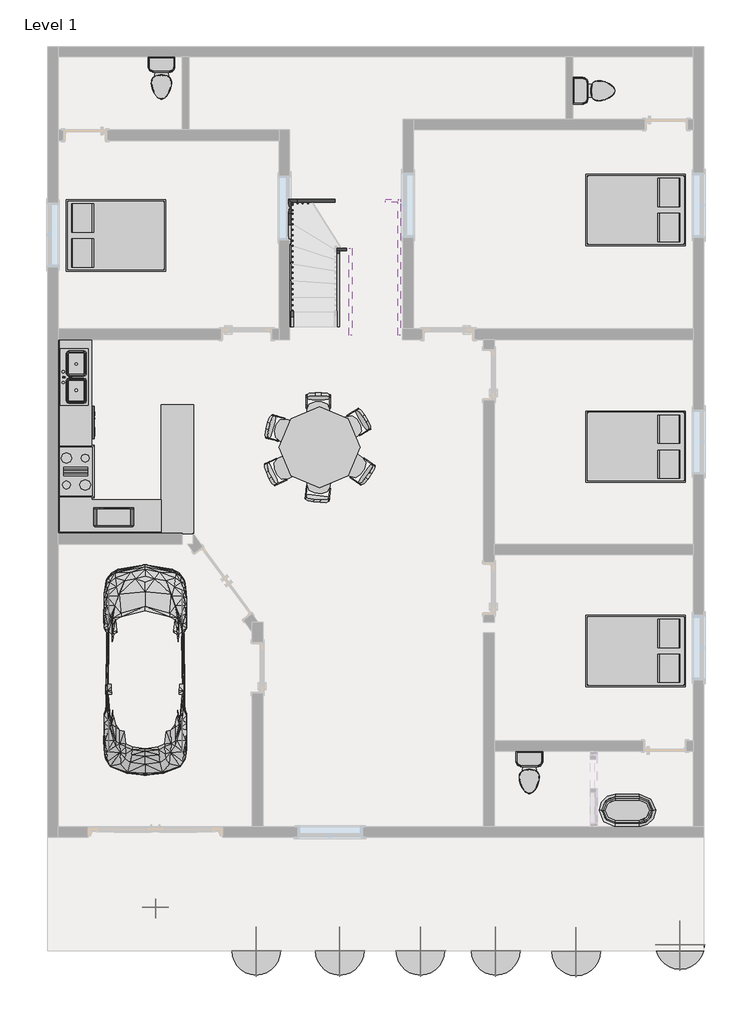
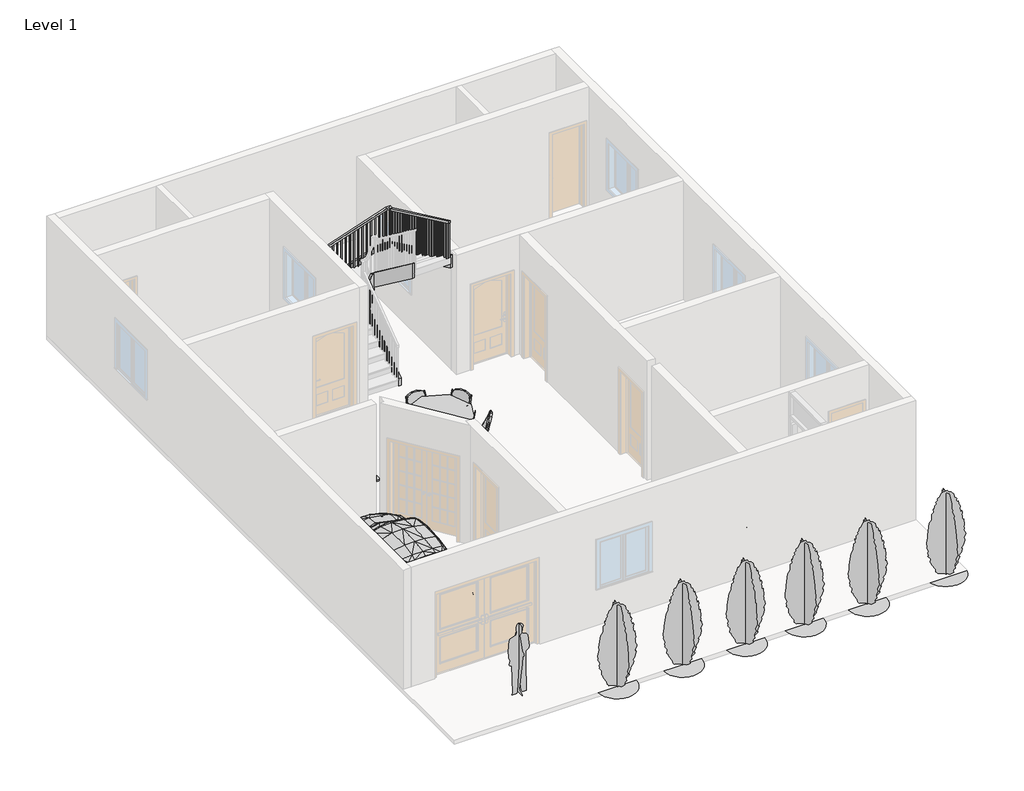
# One storey, part 3 of 3: 13 furniture elements, 9 members, 6 geographic elements, 5 flow terminals, 5 proxies, 1 railing.
"""IFC4 building model written with IfcOpenShell, lengths in millimetres."""

from ifc_helpers import new_model, si_unit, frame, origin, place, context, project, spatial, polyline, outline, extrude, faceted_brep, transform, mapped, element, save
from components import proxy_bb1e6e30, proxy_45b28599, proxy_487063f8, rpc_beetle_rpc_beetle_3ce7ba48, rpc_male_28878092, flow_terminal_a53be723, toilet_domestic_3d_toilet_domestic_3d_f7549cf7, toilet_domestic_3d_toilet_domestic_3d_183bbd19, flow_terminal_f143e1fa, furniture_c8abb964, furniture_15b2fe13, furniture_067af109, furniture_3d1d9cbc, furniture_720490b2, rpc_tree_conifer_chinese_juniper_7_1b9786cd

model = new_model("IFC4")

# Units and contexts
model_context = context("Model", 3, world=origin())
ifc_project = project(units=[si_unit("LENGTHUNIT", "METRE", prefix="MILLI")], contexts=[model_context])

# Site, building, storey
site = spatial("IfcSite", under=ifc_project)
building = spatial("IfcBuilding", under=site)
storey = spatial("IfcBuildingStorey", under=building, Name="Level 1", Elevation=0.0)

# Proxies
placement = place(None, origin())
proxy_shape = proxy_bb1e6e30(model_context)
element("IfcBuildingElementProxy", 1, Name="Cook Top-4 Unit.0001 : 36\" x 20\"", ObjectType="Cook Top-4 Unit.0001 : 36\" x 20\"", at=placement, inside=storey, context=model_context, shape_type="MappedRepresentation", body=[
    mapped(proxy_shape, transform((-2044.8374747, 336.6527309, 152.4), x_axis=(0.0, 1.0, 0.0), y_axis=(-1.0, 0.0, 0.0), z_axis=(0.0, 0.0, 1.0))),
])
proxy_2_shape = proxy_45b28599(model_context)
element("IfcBuildingElementProxy", 2, Name="Dishwasher : 24\" x 24\" x 34\"", ObjectType="Dishwasher : 24\" x 24\" x 34\"", at=placement, inside=storey, context=model_context, shape_type="MappedRepresentation", body=[
    mapped(proxy_2_shape, transform((-1744.7999747, 882.7527309, 0.0), x_axis=(0.0, 1.000000000000002, 0.0), y_axis=(-1.000000000000002, 0.0, 0.0), z_axis=(0.0, 0.0, 1.0))),
])
proxy_3_shape = proxy_487063f8(model_context)
element("IfcBuildingElementProxy", 3, Name="Microwave : 30\" x 16\" x 18\"", ObjectType="Microwave : 30\" x 16\" x 18\"", at=placement, inside=storey, context=model_context, shape_type="MappedRepresentation", body=[
    mapped(proxy_3_shape, transform((-828.5820974, -880.0277749, 0.0), x_axis=(-1.0000000000000004, 0.0, 0.0), y_axis=(0.0, -1.0000000000000004, 0.0), z_axis=(0.0, 0.0, 1.0))),
])
rpc_beetle_rpc_beetle_shape = rpc_beetle_rpc_beetle_3ce7ba48(model_context)
element("IfcBuildingElementProxy", 4, Name="RPC Beetle : RPC Beetle", ObjectType="RPC Beetle : RPC Beetle", at=placement, inside=storey, context=model_context, shape_type="MappedRepresentation", body=[
    mapped(rpc_beetle_rpc_beetle_shape, transform((-731.9749747, -4641.7472691, 0.0), x_axis=(1.0, 0.0, 0.0), y_axis=(0.0, 1.0, 0.0), z_axis=(0.0, 0.0, 1.0))),
])
rpc_male_shape = rpc_male_28878092(model_context)
element("IfcBuildingElementProxy", 5, Name="RPC Male", ObjectType="RPC Male", at=placement, inside=storey, context=model_context, shape_type="MappedRepresentation", body=[
    mapped(rpc_male_shape, transform((-545.8247746, -7892.9472691, 0.0), x_axis=(1.0, 0.0, 0.0), y_axis=(0.0, 1.0, 0.0), z_axis=(0.0, 0.0, 1.0))),
])

# Flow terminals
flow_terminal_shape = flow_terminal_a53be723(model_context)
element("IfcFlowTerminal", 6, ObjectType="Sink Kitchen-Double : 42\" x 21\"", at=placement, inside=storey, context=model_context, shape_type="MappedRepresentation", body=[
    mapped(flow_terminal_shape, transform((-2072.3615606, 2103.7489712, 30.4601563), x_axis=(0.0, 1.0000000000000002, 0.0), y_axis=(-1.0000000000000002, 0.0, 0.0), z_axis=(0.0, 0.0, 1.0))),
])
toilet_domestic_3d_toilet_domestic_3d_shape = toilet_domestic_3d_toilet_domestic_3d_f7549cf7(model_context)
toilet_domestic_3d_toilet_domestic_3d_2_shape = toilet_domestic_3d_toilet_domestic_3d_183bbd19(model_context)
element("IfcFlowTerminal", 7, ObjectType="Toilet-Domestic-3D : Toilet-Domestic-3D", at=placement, inside=storey, context=model_context, shape_type="MappedRepresentation", body=[
    mapped(toilet_domestic_3d_toilet_domestic_3d_shape, transform((-427.1749747, 7674.6817036, 0.0), x_axis=(1.0, 0.0, 0.0), y_axis=(0.0, 1.0, 0.0), z_axis=(0.0, 0.0, 1.0))),
    mapped(toilet_domestic_3d_toilet_domestic_3d_2_shape, transform((-427.1749747, 7674.6817036, 0.0), x_axis=(1.0, 0.0, 0.0), y_axis=(0.0, 1.0, 0.0), z_axis=(0.0, 0.0, 1.0))),
])
element("IfcFlowTerminal", 8, ObjectType="Toilet-Domestic-3D : Toilet-Domestic-3D", at=placement, inside=storey, context=model_context, shape_type="MappedRepresentation", body=[
    mapped(toilet_domestic_3d_toilet_domestic_3d_shape, transform((7839.9210527, 7527.3770127, 0.0), x_axis=(0.0, 1.0000000000000002, 0.0), y_axis=(-1.0000000000000002, 0.0, 0.0), z_axis=(0.0, 0.0, 1.0))),
    mapped(toilet_domestic_3d_toilet_domestic_3d_2_shape, transform((7839.9210527, 7527.3770127, 0.0), x_axis=(0.0, 1.0000000000000002, 0.0), y_axis=(-1.0000000000000002, 0.0, 0.0), z_axis=(0.0, 0.0, 1.0))),
])
element("IfcFlowTerminal", 9, ObjectType="Toilet-Domestic-3D : Toilet-Domestic-3D", at=placement, inside=storey, context=model_context, shape_type="MappedRepresentation", body=[
    mapped(toilet_domestic_3d_toilet_domestic_3d_shape, transform((6524.4875253, -5441.2432964, 0.0), x_axis=(1.0000000000000007, 0.0, 0.0), y_axis=(0.0, 1.0000000000000007, 0.0), z_axis=(0.0, 0.0, 1.0))),
    mapped(toilet_domestic_3d_toilet_domestic_3d_2_shape, transform((6524.4875253, -5441.2432964, 0.0), x_axis=(1.0000000000000007, 0.0, 0.0), y_axis=(0.0, 1.0000000000000007, 0.0), z_axis=(0.0, 0.0, 1.0))),
])
flow_terminal_2_shape = flow_terminal_f143e1fa(model_context)
element("IfcFlowTerminal", 10, ObjectType="Tub-Free Standing-3D : 30\" x 60\"", at=placement, inside=storey, context=model_context, shape_type="MappedRepresentation", body=[
    mapped(flow_terminal_2_shape, transform((8378.6875253, -6064.1472691, 0.0), x_axis=(0.0, 1.0000000000000002, 0.0), y_axis=(-1.0000000000000002, 0.0, 0.0), z_axis=(0.0, 0.0, 1.0))),
])

# Furniture
furniture_shape = furniture_c8abb964(model_context)
element("IfcFurniture", 11, ObjectType="Bed-Box : Double 53\" x 74\"", at=placement, inside=storey, context=model_context, shape_type="MappedRepresentation", body=[
    mapped(furniture_shape, transform((-1522.0294829, 4455.2002719, 0.0), x_axis=(0.0, 1.0, 0.0), y_axis=(-1.0, 0.0, 0.0), z_axis=(0.0, 0.0, 1.0))),
])
element("IfcFurniture", 12, ObjectType="Bed-Box : Double 53\" x 74\"", at=placement, inside=storey, context=model_context, shape_type="MappedRepresentation", body=[
    mapped(furniture_shape, transform((8770.2795335, 5616.10519, 0.0), x_axis=(0.0, -1.0000000000000004, 0.0), y_axis=(1.0000000000000004, 0.0, 0.0), z_axis=(0.0, 0.0, 1.0))),
])
element("IfcFurniture", 13, ObjectType="Bed-Box : Double 53\" x 74\"", at=placement, inside=storey, context=model_context, shape_type="MappedRepresentation", body=[
    mapped(furniture_shape, transform((8770.2795335, 1145.70519, 0.0), x_axis=(0.0, -1.0, 0.0), y_axis=(1.0, 0.0, 0.0), z_axis=(0.0, 0.0, 1.0))),
])
element("IfcFurniture", 14, ObjectType="Bed-Box : Double 53\" x 74\"", at=placement, inside=storey, context=model_context, shape_type="MappedRepresentation", body=[
    mapped(furniture_shape, transform((8770.2795335, -2711.3472691, 0.0), x_axis=(0.0, -1.0, 0.0), y_axis=(1.0, 0.0, 0.0), z_axis=(0.0, 0.0, 1.0))),
])
furniture_2_shape = furniture_15b2fe13(model_context)
element("IfcFurniture", 15, ObjectType="Counter Top-Island.0001 : 48\" Depth", at=placement, inside=storey, context=model_context, shape_type="MappedRepresentation", body=[
    mapped(furniture_2_shape, transform((-406.5374747, 364.407303, 30.4601563), x_axis=(0.0, 1.0000000000000002, 0.0), y_axis=(-1.0000000000000002, 0.0, 0.0), z_axis=(0.0, 0.0, 1.0))),
])
furniture_3_shape = furniture_067af109(model_context)
element("IfcFurniture", 16, ObjectType="Counter Top-L Shaped w Sink : 24\" Depth", at=placement, inside=storey, context=model_context, shape_type="MappedRepresentation", body=[
    mapped(furniture_3_shape, transform((-2379.7999747, 368.715026, 30.4601563), x_axis=(0.0, 1.0000000000000002, 0.0), y_axis=(-1.0000000000000002, 0.0, 0.0), z_axis=(0.0, 0.0, 1.0))),
])
furniture_4_shape = furniture_3d1d9cbc(model_context)
element("IfcFurniture", 17, ObjectType="Seating-Auditorium : 18\" x 24\" x 30\"", at=placement, inside=storey, context=model_context, shape_type="MappedRepresentation", body=[
    mapped(furniture_4_shape, transform((2361.6566068, -123.8075195, 0.0), x_axis=(0.9945218953682721, -0.10452846326766581, 0.0), y_axis=(0.1045284632676658, 0.994521895368272, 0.0), z_axis=(0.0, 0.0, 0.9999999999999999))),
])
element("IfcFurniture", 18, ObjectType="Seating-Auditorium : 18\" x 24\" x 30\"", at=placement, inside=storey, context=model_context, shape_type="MappedRepresentation", body=[
    mapped(furniture_4_shape, transform((3333.5819168, 167.1076408, 0.0), x_axis=(0.5790443741496127, 0.8152960276891364, 0.0), y_axis=(-0.8152960276891364, 0.5790443741496127, 0.0), z_axis=(0.0, 0.0, 1.0))),
])
element("IfcFurniture", 19, ObjectType="Seating-Auditorium : 18\" x 24\" x 30\"", at=placement, inside=storey, context=model_context, shape_type="MappedRepresentation", body=[
    mapped(furniture_4_shape, transform((1606.8827994, 449.404179, 0.0), x_axis=(0.42261826174068884, -0.9063077870366555, 0.0), y_axis=(0.9063077870366555, 0.42261826174068884, 0.0), z_axis=(0.0, 0.0, 1.0))),
])
element("IfcFurniture", 20, ObjectType="Seating-Auditorium : 18\" x 24\" x 30\"", at=placement, inside=storey, context=model_context, shape_type="MappedRepresentation", body=[
    mapped(furniture_4_shape, transform((1704.5988843, 1330.5740196, 0.0), x_axis=(-0.2588190451025253, -0.9659258262890678, 0.0), y_axis=(0.9659258262890678, -0.2588190451025253, 0.0), z_axis=(0.0, 0.0, 1.0))),
])
element("IfcFurniture", 21, ObjectType="Seating-Auditorium : 18\" x 24\" x 30\"", at=placement, inside=storey, context=model_context, shape_type="MappedRepresentation", body=[
    mapped(furniture_4_shape, transform((2697.4913996, 1720.3281408, 0.0), x_axis=(-1.0000000000000004, 0.0, 0.0), y_axis=(0.0, -1.0000000000000004, 0.0), z_axis=(0.0, 0.0, 1.0))),
])
element("IfcFurniture", 22, ObjectType="Seating-Auditorium : 18\" x 24\" x 30\"", at=placement, inside=storey, context=model_context, shape_type="MappedRepresentation", body=[
    mapped(furniture_4_shape, transform((3441.5258387, 1164.5071923, 0.0), x_axis=(-0.515038074910047, 0.8571673007021169, 0.0), y_axis=(-0.8571673007021169, -0.515038074910047, 0.0), z_axis=(0.0, 0.0, 1.0))),
])
furniture_5_shape = furniture_720490b2(model_context)
element("IfcFurniture", 23, ObjectType="Table-Dining Round : 36\" Diameter", at=placement, inside=storey, context=model_context, shape_type="MappedRepresentation", body=[
    mapped(furniture_5_shape, transform((2458.4815635, 978.7314195, 0.0), x_axis=(1.0, 0.0, 0.0), y_axis=(0.0, 1.0, 0.0), z_axis=(0.0, 0.0, 1.0))),
])

# Geographic elements
rpc_tree_conifer_chinese_juniper_7_shape = rpc_tree_conifer_chinese_juniper_7_1b9786cd(model_context)
element("IfcGeographicElement", 24, ObjectType="RPC Tree - Conifer : Chinese Juniper - 7'", at=placement, inside=storey, context=model_context, shape_type="MappedRepresentation", body=[
    mapped(rpc_tree_conifer_chinese_juniper_7_shape, transform((1362.8984947, -8713.8662612, 0.0), x_axis=(1.0, 0.0, 0.0), y_axis=(0.0, 1.0, 0.0), z_axis=(0.0, 0.0, 1.0))),
])
element("IfcGeographicElement", 25, ObjectType="RPC Tree - Conifer : Chinese Juniper - 7'", at=placement, inside=storey, context=model_context, shape_type="MappedRepresentation", body=[
    mapped(rpc_tree_conifer_chinese_juniper_7_shape, transform((2942.5370001, -8713.8662612, 0.0), x_axis=(1.0, 0.0, 0.0), y_axis=(0.0, 1.0, 0.0), z_axis=(0.0, 0.0, 1.0))),
])
element("IfcGeographicElement", 26, ObjectType="RPC Tree - Conifer : Chinese Juniper - 7'", at=placement, inside=storey, context=model_context, shape_type="MappedRepresentation", body=[
    mapped(rpc_tree_conifer_chinese_juniper_7_shape, transform((4466.5370001, -8713.8662612, 0.0), x_axis=(1.0, 0.0, 0.0), y_axis=(0.0, 1.0, 0.0), z_axis=(0.0, 0.0, 1.0))),
])
element("IfcGeographicElement", 27, ObjectType="RPC Tree - Conifer : Chinese Juniper - 7'", at=placement, inside=storey, context=model_context, shape_type="MappedRepresentation", body=[
    mapped(rpc_tree_conifer_chinese_juniper_7_shape, transform((5888.8609947, -8713.8662612, 0.0), x_axis=(1.0, 0.0, 0.0), y_axis=(0.0, 1.0, 0.0), z_axis=(0.0, 0.0, 1.0))),
])
element("IfcGeographicElement", 28, ObjectType="RPC Tree - Conifer : Chinese Juniper - 7'", at=placement, inside=storey, context=model_context, shape_type="MappedRepresentation", body=[
    mapped(rpc_tree_conifer_chinese_juniper_7_shape, transform((7408.0984947, -8726.5662612, 0.0), x_axis=(1.0, 0.0, 0.0), y_axis=(0.0, 1.0, 0.0), z_axis=(0.0, 0.0, 1.0))),
])
element("IfcGeographicElement", 29, ObjectType="RPC Tree - Conifer : Chinese Juniper - 7'", at=placement, inside=storey, context=model_context, shape_type="MappedRepresentation", body=[
    mapped(rpc_tree_conifer_chinese_juniper_7_shape, transform((9373.8533542, -8604.1472691, 0.0), x_axis=(1.0, 0.0, 0.0), y_axis=(0.0, 1.0, 0.0), z_axis=(0.0, 0.0, 1.0))),
])

# Members
element("IfcMember", 30, ObjectType="Stringer - 2\" Width", at=placement, inside=storey, context=model_context, shape_type="SweptSolid", body=[
    extrude(outline(polyline([(3072.6312797, 0.0), (3072.6312797, 232.398685), (5208.4593502, 1303.9014854), (5208.4593502, 962.8953794), (3289.118608, 0.0), (3072.6312797, 0.0)])), frame((1972.130644, 0.0, 0.0), z_axis=(1.0, 0.0, 0.0), x_axis=(0.0, 1.0, 0.0)), (0.0, 0.0, 1.0), 50.8),
])
element("IfcMember", 31, ObjectType="Stringer - 2\" Width", at=placement, inside=storey, context=model_context, shape_type="SweptSolid", body=[
    extrude(outline(polyline([(2022.930644, 5208.4593502), (1972.130644, 5208.4593502), (1972.130644, 5476.6753925), (2022.930644, 5425.8753925), (2022.930644, 5208.4593502)])), frame((0.0, 0.0, 962.8953794), z_axis=(0.0, 0.0, 1.0), x_axis=(1.0, 0.0, 0.0)), (0.0, 0.0, 1.0), 341.0061061),
])
element("IfcMember", 32, ObjectType="Stringer - 2\" Width", at=placement, inside=storey, context=model_context, shape_type="SweptSolid", body=[
    extrude(outline(polyline([(2022.930644, 5425.8753925), (1972.130644, 5476.6753925), (2138.7748321, 5476.6753925), (2138.7748321, 5425.8753925), (2022.930644, 5425.8753925)])), frame((0.0, 0.0, 962.8953794), z_axis=(0.0, 0.0, 1.0), x_axis=(1.0, 0.0, 0.0)), (0.0, 0.0, 1.0), 341.0061061),
])
element("IfcMember", 33, ObjectType="Stringer - 2\" Width", at=placement, inside=storey, context=model_context, shape_type="SweptSolid", body=[
    extrude(outline(polyline([(1303.9014854, 2138.7748321), (962.8953794, 2138.7748321), (1520.4284152, 3810.0442363), (1861.4345213, 3810.0442363), (1303.9014854, 2138.7748321)])), frame((0.0, 5425.8753925, 0.0), z_axis=(0.0, 1.0, 0.0), x_axis=(0.0, 0.0, 1.0)), (0.0, 0.0, 1.0), 50.8),
])
element("IfcMember", 34, ObjectType="Stringer - 2\" Width", at=placement, inside=storey, context=model_context, shape_type="SweptSolid", body=[
    extrude(outline(polyline([(3810.0442363, 5425.8753925), (3810.0442363, 5476.6753925), (4040.1107574, 5476.6753925), (4040.1107574, 5425.8753925), (3810.0442363, 5425.8753925)])), frame((0.0, 0.0, 1529.8677443), z_axis=(0.0, 0.0, 1.0), x_axis=(1.0, 0.0, 0.0)), (0.0, 0.0, 1.0), 321.3129818),
])
element("IfcMember", 35, ObjectType="Stringer - 2\" Width", at=placement, inside=storey, context=model_context, shape_type="SweptSolid", body=[
    extrude(outline(polyline([(3072.6312797, 0.0), (3072.6312797, 189.3921594), (4506.1853358, 1242.3151337), (4506.1853358, 864.1337167), (3329.6677512, 0.0), (3072.6312797, 0.0)])), frame((2891.8207007, 0.0, 0.0), z_axis=(1.0, 0.0, 0.0), x_axis=(0.0, 1.0, 0.0)), (0.0, 0.0, 1.0), 50.8),
])
element("IfcMember", 36, ObjectType="Stringer - 2\" Width", at=placement, inside=storey, context=model_context, shape_type="SweptSolid", body=[
    extrude(outline(polyline([(1530.2439876, 2891.8207007), (901.4455201, 2891.8207007), (901.4455201, 2934.2339989), (1299.5579895, 3120.4207007), (1913.6276378, 3120.4207007), (1913.6276378, 3071.1191222), (1530.2439876, 2891.8207007)])), frame((0.0, 4506.1853358, 0.0), z_axis=(0.0, 1.0, 0.0), x_axis=(0.0, 0.0, 1.0)), (0.0, 0.0, 1.0), 50.8),
])
element("IfcMember", 37, ObjectType="Stringer - 2\" Width", at=placement, inside=storey, context=model_context, shape_type="SweptSolid", body=[
    extrude(outline(polyline([(4556.9853358, 1913.6276378), (4556.9853358, 1532.6570539), (2913.6927876, 2764.8621246), (2913.6927876, 3145.8327085), (4556.9853358, 1913.6276378)])), frame((3120.4207007, 0.0, 0.0), z_axis=(1.0, 0.0, 0.0), x_axis=(0.0, 1.0, 0.0)), (0.0, 0.0, 1.0), 50.8),
])
element("IfcMember", 38, ObjectType="Stringer - 2\" Width", at=placement, inside=storey, context=model_context, shape_type="SweptSolid", body=[
    extrude(outline(polyline([(5476.6753925, 1827.2654608), (5476.6753925, 1546.3807261), (5390.7990734, 1546.3807261), (2913.6927876, 2712.5353345), (2913.6927876, 3033.8483163), (5476.6753925, 1827.2654608)])), frame((4040.1107574, 0.0, 0.0), z_axis=(1.0, 0.0, 0.0), x_axis=(0.0, 1.0, 0.0)), (0.0, 0.0, 1.0), 50.8),
])

# Railing
element("IfcRailing", 39, ObjectType="Handrail - Rectangular", at=placement, inside=storey, context=model_context, shape_type="SolidModel", body=[
    faceted_brep([(2022.930644, 3072.6312797, 1112.8971996), (2022.930644, 3072.6312797, 1056.0628486), (2073.730644, 3072.6312797, 1056.0628486), (2073.730644, 3072.6312797, 1112.8971996), (2022.930644, 5274.3963768, 2217.4793052), (2022.930644, 5286.4246574, 2166.6793052), (2073.730644, 5286.4246574, 2166.6793052), (2073.730644, 5274.3963768, 2217.4793052), (2022.930644, 5425.8753925, 2166.6793052), (2022.930644, 5425.8753925, 2217.4793052), (2237.9338544, 5425.8753925, 2217.4793052), (2246.1837815, 5425.8753925, 2166.6793052), (2073.730644, 5375.0753925, 2166.6793052), (2246.1837815, 5375.0753925, 2166.6793052), (2073.730644, 5375.0753925, 2217.4793052), (2237.9338544, 5375.0753925, 2217.4793052), (4040.1107574, 5425.8753925, 2731.2500787), (4040.1107574, 5425.8753925, 2782.0500787), (4040.1107574, 5340.6601233, 2782.0500787), (4040.1107574, 5329.3004223, 2731.2500787), (3989.3107574, 5375.0753925, 2731.2500787), (3989.3107574, 5329.3004223, 2731.2500787), (3989.3107574, 5375.0753925, 2782.0500787), (3989.3107574, 5340.6601233, 2782.0500787), (3930.2996865, 5425.8753925, 2782.0500787), (3938.5496136, 5425.8753925, 2731.2500787), (3938.5496136, 5375.0753925, 2731.2500787), (3930.2996865, 5375.0753925, 2782.0500787), (4040.1107574, 2913.6927876, 3924.600626), (3989.3107574, 2913.6927876, 3924.600626), (3989.3107574, 2913.6927876, 3868.4527862), (4040.1107574, 2913.6927876, 3868.4527862)], [[[0, 1, 2, 3]], [[1, 0, 4, 5]], [[2, 1, 5, 6]], [[3, 2, 6, 7]], [[0, 3, 7, 4]], [[8, 9, 10, 11]], [[12, 8, 11, 13]], [[14, 12, 13, 15]], [[9, 14, 15, 10]], [[16, 17, 18, 19]], [[20, 16, 19, 21]], [[22, 20, 21, 23]], [[17, 22, 23, 18]], [[5, 4, 9, 8]], [[6, 5, 8, 12]], [[7, 6, 12, 14]], [[4, 7, 14, 9]], [[11, 10, 24, 25]], [[13, 11, 25, 26]], [[15, 13, 26, 27]], [[10, 15, 27, 24]], [[25, 24, 17, 16]], [[26, 25, 16, 20]], [[27, 26, 20, 22]], [[24, 27, 22, 17]], [[28, 29, 30, 31]], [[19, 18, 28, 31]], [[21, 19, 31, 30]], [[23, 21, 30, 29]], [[18, 23, 29, 28]]]),
    extrude(outline(polyline([(3013.3851233, 3821.5203323), (3013.3851233, 2878.6666667), (2994.3351233, 2878.6666667), (2994.3351233, 3830.4885568), (3013.3851233, 3821.5203323)])), frame((4005.1857574, 0.0, 0.0), z_axis=(1.0, 0.0, 0.0), x_axis=(0.0, 1.0, 0.0)), (0.0, 0.0, 1.0), 19.05),
    extrude(outline(polyline([(3114.9851233, 3773.6898016), (3114.9851233, 2878.6666667), (3095.9351233, 2878.6666667), (3095.9351233, 3782.6580261), (3114.9851233, 3773.6898016)])), frame((4005.1857574, 0.0, 0.0), z_axis=(1.0, 0.0, 0.0), x_axis=(0.0, 1.0, 0.0)), (0.0, 0.0, 1.0), 19.05),
    extrude(outline(polyline([(3216.5851233, 3725.8592709), (3216.5851233, 2709.3333333), (3197.5351233, 2709.3333333), (3197.5351233, 3734.8274954), (3216.5851233, 3725.8592709)])), frame((4005.1857574, 0.0, 0.0), z_axis=(1.0, 0.0, 0.0), x_axis=(0.0, 1.0, 0.0)), (0.0, 0.0, 1.0), 19.05),
    extrude(outline(polyline([(3318.1851233, 3678.0287402), (3318.1851233, 2709.3333333), (3299.1351233, 2709.3333333), (3299.1351233, 3686.9969647), (3318.1851233, 3678.0287402)])), frame((4005.1857574, 0.0, 0.0), z_axis=(1.0, 0.0, 0.0), x_axis=(0.0, 1.0, 0.0)), (0.0, 0.0, 1.0), 19.05),
    extrude(outline(polyline([(3419.7851233, 3630.1982096), (3419.7851233, 2709.3333333), (3400.7351233, 2709.3333333), (3400.7351233, 3639.1664341), (3419.7851233, 3630.1982096)])), frame((4005.1857574, 0.0, 0.0), z_axis=(1.0, 0.0, 0.0), x_axis=(0.0, 1.0, 0.0)), (0.0, 0.0, 1.0), 19.05),
    extrude(outline(polyline([(3521.3851233, 3582.3676789), (3521.3851233, 2540.0), (3502.3351233, 2540.0), (3502.3351233, 3591.3359034), (3521.3851233, 3582.3676789)])), frame((4005.1857574, 0.0, 0.0), z_axis=(1.0, 0.0, 0.0), x_axis=(0.0, 1.0, 0.0)), (0.0, 0.0, 1.0), 19.05),
    extrude(outline(polyline([(3622.9851233, 3534.5371482), (3622.9851233, 2540.0), (3603.9351233, 2540.0), (3603.9351233, 3543.5053727), (3622.9851233, 3534.5371482)])), frame((4005.1857574, 0.0, 0.0), z_axis=(1.0, 0.0, 0.0), x_axis=(0.0, 1.0, 0.0)), (0.0, 0.0, 1.0), 19.05),
    extrude(outline(polyline([(3724.5851233, 3486.7066175), (3724.5851233, 2540.0), (3705.5351233, 2540.0), (3705.5351233, 3495.674842), (3724.5851233, 3486.7066175)])), frame((4005.1857574, 0.0, 0.0), z_axis=(1.0, 0.0, 0.0), x_axis=(0.0, 1.0, 0.0)), (0.0, 0.0, 1.0), 19.05),
    extrude(outline(polyline([(3826.1851233, 3438.8760868), (3826.1851233, 2370.6666667), (3807.1351233, 2370.6666667), (3807.1351233, 3447.8443113), (3826.1851233, 3438.8760868)])), frame((4005.1857574, 0.0, 0.0), z_axis=(1.0, 0.0, 0.0), x_axis=(0.0, 1.0, 0.0)), (0.0, 0.0, 1.0), 19.05),
    extrude(outline(polyline([(3927.7851233, 3391.0455561), (3927.7851233, 2370.6666667), (3908.7351233, 2370.6666667), (3908.7351233, 3400.0137806), (3927.7851233, 3391.0455561)])), frame((4005.1857574, 0.0, 0.0), z_axis=(1.0, 0.0, 0.0), x_axis=(0.0, 1.0, 0.0)), (0.0, 0.0, 1.0), 19.05),
    extrude(outline(polyline([(4029.3851233, 3343.2150255), (4029.3851233, 2370.6666667), (4010.3351233, 2370.6666667), (4010.3351233, 3352.18325), (4029.3851233, 3343.2150255)])), frame((4005.1857574, 0.0, 0.0), z_axis=(1.0, 0.0, 0.0), x_axis=(0.0, 1.0, 0.0)), (0.0, 0.0, 1.0), 19.05),
    extrude(outline(polyline([(4130.9851233, 3295.3844948), (4130.9851233, 2201.3333333), (4111.9351233, 2201.3333333), (4111.9351233, 3304.3527193), (4130.9851233, 3295.3844948)])), frame((4005.1857574, 0.0, 0.0), z_axis=(1.0, 0.0, 0.0), x_axis=(0.0, 1.0, 0.0)), (0.0, 0.0, 1.0), 19.05),
    extrude(outline(polyline([(4232.5851233, 3247.5539641), (4232.5851233, 2201.3333333), (4213.5351233, 2201.3333333), (4213.5351233, 3256.5221886), (4232.5851233, 3247.5539641)])), frame((4005.1857574, 0.0, 0.0), z_axis=(1.0, 0.0, 0.0), x_axis=(0.0, 1.0, 0.0)), (0.0, 0.0, 1.0), 19.05),
    extrude(outline(polyline([(4334.1851233, 3199.7234334), (4334.1851233, 2201.3333333), (4315.1351233, 2201.3333333), (4315.1351233, 3208.6916579), (4334.1851233, 3199.7234334)])), frame((4005.1857574, 0.0, 0.0), z_axis=(1.0, 0.0, 0.0), x_axis=(0.0, 1.0, 0.0)), (0.0, 0.0, 1.0), 19.05),
    extrude(outline(polyline([(4435.7851233, 3151.8929027), (4435.7851233, 2032.0), (4416.7351233, 2032.0), (4416.7351233, 3160.8611272), (4435.7851233, 3151.8929027)])), frame((4005.1857574, 0.0, 0.0), z_axis=(1.0, 0.0, 0.0), x_axis=(0.0, 1.0, 0.0)), (0.0, 0.0, 1.0), 19.05),
    extrude(outline(polyline([(4537.3851233, 3104.062372), (4537.3851233, 2032.0), (4518.3351233, 2032.0), (4518.3351233, 3113.0305966), (4537.3851233, 3104.062372)])), frame((4005.1857574, 0.0, 0.0), z_axis=(1.0, 0.0, 0.0), x_axis=(0.0, 1.0, 0.0)), (0.0, 0.0, 1.0), 19.05),
    extrude(outline(polyline([(4638.9851233, 3056.2318414), (4638.9851233, 2032.0), (4619.9351233, 2032.0), (4619.9351233, 3065.2000659), (4638.9851233, 3056.2318414)])), frame((4005.1857574, 0.0, 0.0), z_axis=(1.0, 0.0, 0.0), x_axis=(0.0, 1.0, 0.0)), (0.0, 0.0, 1.0), 19.05),
    extrude(outline(polyline([(4740.5851233, 3008.4013107), (4740.5851233, 2032.0), (4721.5351233, 2032.0), (4721.5351233, 3017.3695352), (4740.5851233, 3008.4013107)])), frame((4005.1857574, 0.0, 0.0), z_axis=(1.0, 0.0, 0.0), x_axis=(0.0, 1.0, 0.0)), (0.0, 0.0, 1.0), 19.05),
    extrude(outline(polyline([(4842.1851233, 2960.57078), (4842.1851233, 1862.6666667), (4823.1351233, 1862.6666667), (4823.1351233, 2969.5390045), (4842.1851233, 2960.57078)])), frame((4005.1857574, 0.0, 0.0), z_axis=(1.0, 0.0, 0.0), x_axis=(0.0, 1.0, 0.0)), (0.0, 0.0, 1.0), 19.05),
    extrude(outline(polyline([(4943.7851233, 2912.7402493), (4943.7851233, 1862.6666667), (4924.7351233, 1862.6666667), (4924.7351233, 2921.7084738), (4943.7851233, 2912.7402493)])), frame((4005.1857574, 0.0, 0.0), z_axis=(1.0, 0.0, 0.0), x_axis=(0.0, 1.0, 0.0)), (0.0, 0.0, 1.0), 19.05),
    extrude(outline(polyline([(5045.3851233, 2864.9097186), (5045.3851233, 1862.6666667), (5026.3351233, 1862.6666667), (5026.3351233, 2873.8779431), (5045.3851233, 2864.9097186)])), frame((4005.1857574, 0.0, 0.0), z_axis=(1.0, 0.0, 0.0), x_axis=(0.0, 1.0, 0.0)), (0.0, 0.0, 1.0), 19.05),
    extrude(outline(polyline([(5146.9851233, 2817.079188), (5146.9851233, 1862.6666667), (5127.9351233, 1862.6666667), (5127.9351233, 2826.0474125), (5146.9851233, 2817.079188)])), frame((4005.1857574, 0.0, 0.0), z_axis=(1.0, 0.0, 0.0), x_axis=(0.0, 1.0, 0.0)), (0.0, 0.0, 1.0), 19.05),
    extrude(outline(polyline([(5248.5851233, 2769.2486573), (5248.5851233, 1862.6666667), (5229.5351233, 1862.6666667), (5229.5351233, 2778.2168818), (5248.5851233, 2769.2486573)])), frame((4005.1857574, 0.0, 0.0), z_axis=(1.0, 0.0, 0.0), x_axis=(0.0, 1.0, 0.0)), (0.0, 0.0, 1.0), 19.05),
    extrude(outline(polyline([(2702.9126789, 3854.0088544), (1693.3333333, 3854.0088544), (1693.3333333, 3873.0588544), (2709.2677311, 3873.0588544), (2702.9126789, 3854.0088544)])), frame((0.0, 5390.9503925, 0.0), z_axis=(0.0, 1.0, 0.0), x_axis=(0.0, 0.0, 1.0)), (0.0, 0.0, 1.0), 19.05),
    extrude(outline(polyline([(2669.1537929, 3752.4088544), (1693.3333333, 3752.4088544), (1693.3333333, 3771.4588544), (2675.5088451, 3771.4588544), (2669.1537929, 3752.4088544)])), frame((0.0, 5390.9503925, 0.0), z_axis=(0.0, 1.0, 0.0), x_axis=(0.0, 0.0, 1.0)), (0.0, 0.0, 1.0), 19.05),
    extrude(outline(polyline([(2635.260181, 3650.8088544), (1693.3333333, 3650.8088544), (1693.3333333, 3669.8588544), (2641.6152333, 3669.8588544), (2635.260181, 3650.8088544)])), frame((0.0, 5390.9503925, 0.0), z_axis=(0.0, 1.0, 0.0), x_axis=(0.0, 0.0, 1.0)), (0.0, 0.0, 1.0), 19.05),
    extrude(outline(polyline([(2601.3665692, 3549.2088544), (1693.3333333, 3549.2088544), (1693.3333333, 3568.2588544), (2607.7216214, 3568.2588544), (2601.3665692, 3549.2088544)])), frame((0.0, 5390.9503925, 0.0), z_axis=(0.0, 1.0, 0.0), x_axis=(0.0, 0.0, 1.0)), (0.0, 0.0, 1.0), 19.05),
    extrude(outline(polyline([(2567.4729574, 3447.6088544), (1693.3333333, 3447.6088544), (1693.3333333, 3466.6588544), (2573.8280096, 3466.6588544), (2567.4729574, 3447.6088544)])), frame((0.0, 5390.9503925, 0.0), z_axis=(0.0, 1.0, 0.0), x_axis=(0.0, 0.0, 1.0)), (0.0, 0.0, 1.0), 19.05),
    extrude(outline(polyline([(2533.5793456, 3346.0088544), (1524.0, 3346.0088544), (1524.0, 3365.0588544), (2539.9343978, 3365.0588544), (2533.5793456, 3346.0088544)])), frame((0.0, 5390.9503925, 0.0), z_axis=(0.0, 1.0, 0.0), x_axis=(0.0, 0.0, 1.0)), (0.0, 0.0, 1.0), 19.05),
    extrude(outline(polyline([(2499.8204595, 3244.4088544), (1524.0, 3244.4088544), (1524.0, 3263.4588544), (2506.1755117, 3263.4588544), (2499.8204595, 3244.4088544)])), frame((0.0, 5390.9503925, 0.0), z_axis=(0.0, 1.0, 0.0), x_axis=(0.0, 0.0, 1.0)), (0.0, 0.0, 1.0), 19.05),
    extrude(outline(polyline([(2465.9268477, 3142.8088544), (1524.0, 3142.8088544), (1524.0, 3161.8588544), (2472.2818999, 3161.8588544), (2465.9268477, 3142.8088544)])), frame((0.0, 5390.9503925, 0.0), z_axis=(0.0, 1.0, 0.0), x_axis=(0.0, 0.0, 1.0)), (0.0, 0.0, 1.0), 19.05),
    extrude(outline(polyline([(2432.0332359, 3041.2088544), (1524.0, 3041.2088544), (1524.0, 3060.2588544), (2438.3882881, 3060.2588544), (2432.0332359, 3041.2088544)])), frame((0.0, 5390.9503925, 0.0), z_axis=(0.0, 1.0, 0.0), x_axis=(0.0, 0.0, 1.0)), (0.0, 0.0, 1.0), 19.05),
    extrude(outline(polyline([(2398.1396241, 2939.6088544), (1524.0, 2939.6088544), (1524.0, 2958.6588544), (2404.4946763, 2958.6588544), (2398.1396241, 2939.6088544)])), frame((0.0, 5390.9503925, 0.0), z_axis=(0.0, 1.0, 0.0), x_axis=(0.0, 0.0, 1.0)), (0.0, 0.0, 1.0), 19.05),
    extrude(outline(polyline([(2364.2460122, 2838.0088544), (1354.6666667, 2838.0088544), (1354.6666667, 2857.0588544), (2370.6010644, 2857.0588544), (2364.2460122, 2838.0088544)])), frame((0.0, 5390.9503925, 0.0), z_axis=(0.0, 1.0, 0.0), x_axis=(0.0, 0.0, 1.0)), (0.0, 0.0, 1.0), 19.05),
    extrude(outline(polyline([(2330.2176746, 2736.4088544), (1354.6666667, 2736.4088544), (1354.6666667, 2755.4588544), (2336.5727268, 2755.4588544), (2330.2176746, 2736.4088544)])), frame((0.0, 5390.9503925, 0.0), z_axis=(0.0, 1.0, 0.0), x_axis=(0.0, 0.0, 1.0)), (0.0, 0.0, 1.0), 19.05),
    extrude(outline(polyline([(2296.3240628, 2634.8088544), (1354.6666667, 2634.8088544), (1354.6666667, 2653.8588544), (2302.679115, 2653.8588544), (2296.3240628, 2634.8088544)])), frame((0.0, 5390.9503925, 0.0), z_axis=(0.0, 1.0, 0.0), x_axis=(0.0, 0.0, 1.0)), (0.0, 0.0, 1.0), 19.05),
    extrude(outline(polyline([(2262.430451, 2533.2088544), (1354.6666667, 2533.2088544), (1354.6666667, 2552.2588544), (2268.7855032, 2552.2588544), (2262.430451, 2533.2088544)])), frame((0.0, 5390.9503925, 0.0), z_axis=(0.0, 1.0, 0.0), x_axis=(0.0, 0.0, 1.0)), (0.0, 0.0, 1.0), 19.05),
    extrude(outline(polyline([(2228.5368391, 2431.6088544), (1354.6666667, 2431.6088544), (1354.6666667, 2450.6588544), (2234.8918914, 2450.6588544), (2228.5368391, 2431.6088544)])), frame((0.0, 5390.9503925, 0.0), z_axis=(0.0, 1.0, 0.0), x_axis=(0.0, 0.0, 1.0)), (0.0, 0.0, 1.0), 19.05),
    extrude(outline(polyline([(2194.6432273, 2330.0088544), (1185.3333333, 2330.0088544), (1185.3333333, 2349.0588544), (2200.9982795, 2349.0588544), (2194.6432273, 2330.0088544)])), frame((0.0, 5390.9503925, 0.0), z_axis=(0.0, 1.0, 0.0), x_axis=(0.0, 0.0, 1.0)), (0.0, 0.0, 1.0), 19.05),
    extrude(outline(polyline([(2140.405644, 5410.0003925), (2159.455644, 5410.0003925), (2159.455644, 5390.9503925), (2140.405644, 5390.9503925), (2140.405644, 5410.0003925)])), frame((0.0, 0.0, 1185.3333333), z_axis=(0.0, 0.0, 1.0), x_axis=(1.0, 0.0, 0.0)), (0.0, 0.0, 1.0), 981.3459719),
    extrude(outline(polyline([(2038.805644, 5366.4713768), (2038.805644, 5385.5213768), (2057.855644, 5385.5213768), (2057.855644, 5366.4713768), (2038.805644, 5366.4713768)])), frame((0.0, 0.0, 1185.3333333), z_axis=(0.0, 0.0, 1.0), x_axis=(1.0, 0.0, 0.0)), (0.0, 0.0, 1.0), 981.3459719),
    extrude(outline(polyline([(5215.7562797, 2131.2263745), (5215.7562797, 1185.3333333), (5196.7062797, 1185.3333333), (5196.7062797, 2121.6693654), (5215.7562797, 2131.2263745)])), frame((2038.805644, 0.0, 0.0), z_axis=(1.0, 0.0, 0.0), x_axis=(0.0, 1.0, 0.0)), (0.0, 0.0, 1.0), 19.05),
    extrude(outline(polyline([(5114.1562797, 2080.2556592), (5114.1562797, 1185.3333333), (5095.1062797, 1185.3333333), (5095.1062797, 2070.6986501), (5114.1562797, 2080.2556592)])), frame((2038.805644, 0.0, 0.0), z_axis=(1.0, 0.0, 0.0), x_axis=(0.0, 1.0, 0.0)), (0.0, 0.0, 1.0), 19.05),
    extrude(outline(polyline([(5012.5562797, 2029.2849439), (5012.5562797, 1016.0), (4993.5062797, 1016.0), (4993.5062797, 2019.7279348), (5012.5562797, 2029.2849439)])), frame((2038.805644, 0.0, 0.0), z_axis=(1.0, 0.0, 0.0), x_axis=(0.0, 1.0, 0.0)), (0.0, 0.0, 1.0), 19.05),
    extrude(outline(polyline([(4910.9562797, 1978.3142286), (4910.9562797, 1016.0), (4891.9062797, 1016.0), (4891.9062797, 1968.7572195), (4910.9562797, 1978.3142286)])), frame((2038.805644, 0.0, 0.0), z_axis=(1.0, 0.0, 0.0), x_axis=(0.0, 1.0, 0.0)), (0.0, 0.0, 1.0), 19.05),
    extrude(outline(polyline([(4809.3562797, 1927.3435133), (4809.3562797, 1016.0), (4790.3062797, 1016.0), (4790.3062797, 1917.7865042), (4809.3562797, 1927.3435133)])), frame((2038.805644, 0.0, 0.0), z_axis=(1.0, 0.0, 0.0), x_axis=(0.0, 1.0, 0.0)), (0.0, 0.0, 1.0), 19.05),
    extrude(outline(polyline([(4707.7562797, 1876.372798), (4707.7562797, 1016.0), (4688.7062797, 1016.0), (4688.7062797, 1866.8157889), (4707.7562797, 1876.372798)])), frame((2038.805644, 0.0, 0.0), z_axis=(1.0, 0.0, 0.0), x_axis=(0.0, 1.0, 0.0)), (0.0, 0.0, 1.0), 19.05),
    extrude(outline(polyline([(4606.1562797, 1825.4020827), (4606.1562797, 846.6666667), (4587.1062797, 846.6666667), (4587.1062797, 1815.8450736), (4606.1562797, 1825.4020827)])), frame((2038.805644, 0.0, 0.0), z_axis=(1.0, 0.0, 0.0), x_axis=(0.0, 1.0, 0.0)), (0.0, 0.0, 1.0), 19.05),
    extrude(outline(polyline([(4504.5562797, 1774.4313674), (4504.5562797, 846.6666667), (4485.5062797, 846.6666667), (4485.5062797, 1764.8743583), (4504.5562797, 1774.4313674)])), frame((2038.805644, 0.0, 0.0), z_axis=(1.0, 0.0, 0.0), x_axis=(0.0, 1.0, 0.0)), (0.0, 0.0, 1.0), 19.05),
    extrude(outline(polyline([(4402.9562797, 1723.4606521), (4402.9562797, 846.6666667), (4383.9062797, 846.6666667), (4383.9062797, 1713.903643), (4402.9562797, 1723.4606521)])), frame((2038.805644, 0.0, 0.0), z_axis=(1.0, 0.0, 0.0), x_axis=(0.0, 1.0, 0.0)), (0.0, 0.0, 1.0), 19.05),
    extrude(outline(polyline([(4301.3562797, 1672.4899368), (4301.3562797, 846.6666667), (4282.3062797, 846.6666667), (4282.3062797, 1662.9329277), (4301.3562797, 1672.4899368)])), frame((2038.805644, 0.0, 0.0), z_axis=(1.0, 0.0, 0.0), x_axis=(0.0, 1.0, 0.0)), (0.0, 0.0, 1.0), 19.05),
    extrude(outline(polyline([(4199.7562797, 1621.5192215), (4199.7562797, 677.3333333), (4180.7062797, 677.3333333), (4180.7062797, 1611.9622124), (4199.7562797, 1621.5192215)])), frame((2038.805644, 0.0, 0.0), z_axis=(1.0, 0.0, 0.0), x_axis=(0.0, 1.0, 0.0)), (0.0, 0.0, 1.0), 19.05),
    extrude(outline(polyline([(4098.1562797, 1570.5485062), (4098.1562797, 677.3333333), (4079.1062797, 677.3333333), (4079.1062797, 1560.9914971), (4098.1562797, 1570.5485062)])), frame((2038.805644, 0.0, 0.0), z_axis=(1.0, 0.0, 0.0), x_axis=(0.0, 1.0, 0.0)), (0.0, 0.0, 1.0), 19.05),
    extrude(outline(polyline([(3996.5562797, 1519.5777909), (3996.5562797, 677.3333333), (3977.5062797, 677.3333333), (3977.5062797, 1510.0207818), (3996.5562797, 1519.5777909)])), frame((2038.805644, 0.0, 0.0), z_axis=(1.0, 0.0, 0.0), x_axis=(0.0, 1.0, 0.0)), (0.0, 0.0, 1.0), 19.05),
    extrude(outline(polyline([(3894.9562797, 1468.6070756), (3894.9562797, 508.0), (3875.9062797, 508.0), (3875.9062797, 1459.0500664), (3894.9562797, 1468.6070756)])), frame((2038.805644, 0.0, 0.0), z_axis=(1.0, 0.0, 0.0), x_axis=(0.0, 1.0, 0.0)), (0.0, 0.0, 1.0), 19.05),
    extrude(outline(polyline([(3793.3562797, 1417.6363603), (3793.3562797, 508.0), (3774.3062797, 508.0), (3774.3062797, 1408.0793511), (3793.3562797, 1417.6363603)])), frame((2038.805644, 0.0, 0.0), z_axis=(1.0, 0.0, 0.0), x_axis=(0.0, 1.0, 0.0)), (0.0, 0.0, 1.0), 19.05),
    extrude(outline(polyline([(3691.7562797, 1366.665645), (3691.7562797, 508.0), (3672.7062797, 508.0), (3672.7062797, 1357.1086358), (3691.7562797, 1366.665645)])), frame((2038.805644, 0.0, 0.0), z_axis=(1.0, 0.0, 0.0), x_axis=(0.0, 1.0, 0.0)), (0.0, 0.0, 1.0), 19.05),
    extrude(outline(polyline([(3590.1562797, 1315.6949297), (3590.1562797, 338.6666667), (3571.1062797, 338.6666667), (3571.1062797, 1306.1379205), (3590.1562797, 1315.6949297)])), frame((2038.805644, 0.0, 0.0), z_axis=(1.0, 0.0, 0.0), x_axis=(0.0, 1.0, 0.0)), (0.0, 0.0, 1.0), 19.05),
    extrude(outline(polyline([(3488.5562797, 1264.7242143), (3488.5562797, 338.6666667), (3469.5062797, 338.6666667), (3469.5062797, 1255.1672052), (3488.5562797, 1264.7242143)])), frame((2038.805644, 0.0, 0.0), z_axis=(1.0, 0.0, 0.0), x_axis=(0.0, 1.0, 0.0)), (0.0, 0.0, 1.0), 19.05),
    extrude(outline(polyline([(3386.9562797, 1213.753499), (3386.9562797, 338.6666667), (3367.9062797, 338.6666667), (3367.9062797, 1204.1964899), (3386.9562797, 1213.753499)])), frame((2038.805644, 0.0, 0.0), z_axis=(1.0, 0.0, 0.0), x_axis=(0.0, 1.0, 0.0)), (0.0, 0.0, 1.0), 19.05),
    extrude(outline(polyline([(3285.3562797, 1162.7827837), (3285.3562797, 169.3333333), (3266.3062797, 169.3333333), (3266.3062797, 1153.2257746), (3285.3562797, 1162.7827837)])), frame((2038.805644, 0.0, 0.0), z_axis=(1.0, 0.0, 0.0), x_axis=(0.0, 1.0, 0.0)), (0.0, 0.0, 1.0), 19.05),
    extrude(outline(polyline([(3183.7562797, 1111.8120684), (3183.7562797, 169.3333333), (3164.7062797, 169.3333333), (3164.7062797, 1102.2550593), (3183.7562797, 1111.8120684)])), frame((2038.805644, 0.0, 0.0), z_axis=(1.0, 0.0, 0.0), x_axis=(0.0, 1.0, 0.0)), (0.0, 0.0, 1.0), 19.05),
    extrude(outline(polyline([(4024.2357574, 5350.1851233), (4024.2357574, 5331.1351233), (4005.1857574, 5331.1351233), (4005.1857574, 5350.1851233), (4024.2357574, 5350.1851233)])), frame((0.0, 0.0, 1693.3333333), z_axis=(0.0, 0.0, 1.0), x_axis=(1.0, 0.0, 0.0)), (0.0, 0.0, 1.0), 1037.9167453),
    extrude(outline(polyline([(4005.1857574, 5410.0003925), (4024.2357574, 5410.0003925), (4024.2357574, 5390.9503925), (4005.1857574, 5390.9503925), (4005.1857574, 5410.0003925)])), frame((0.0, 0.0, 1693.3333333), z_axis=(0.0, 0.0, 1.0), x_axis=(1.0, 0.0, 0.0)), (0.0, 0.0, 1.0), 1037.9167453),
    extrude(outline(polyline([(2725.3203889, 3920.7746865), (1693.3333333, 3920.7746865), (1693.3333333, 3939.8246865), (2731.6754411, 3939.8246865), (2725.3203889, 3920.7746865)])), frame((0.0, 5390.9503925, 0.0), z_axis=(0.0, 1.0, 0.0), x_axis=(0.0, 0.0, 1.0)), (0.0, 0.0, 1.0), 19.05),
    extrude(outline(polyline([(2228.4088544, 5410.0003925), (2247.4588544, 5410.0003925), (2247.4588544, 5390.9503925), (2228.4088544, 5390.9503925), (2228.4088544, 5410.0003925)])), frame((0.0, 0.0, 1185.3333333), z_axis=(0.0, 0.0, 1.0), x_axis=(1.0, 0.0, 0.0)), (0.0, 0.0, 1.0), 981.3459719),
    extrude(outline(polyline([(2038.805644, 5390.9503925), (2038.805644, 5410.0003925), (2057.855644, 5410.0003925), (2057.855644, 5390.9503925), (2038.805644, 5390.9503925)])), frame((0.0, 0.0, 1185.3333333), z_axis=(0.0, 0.0, 1.0), x_axis=(1.0, 0.0, 0.0)), (0.0, 0.0, 1.0), 981.3459719),
    extrude(outline(polyline([(5283.9213768, 2165.4234588), (5283.9213768, 1185.3333333), (5264.8713768, 1185.3333333), (5264.8713768, 2155.8664497), (5283.9213768, 2165.4234588)])), frame((2038.805644, 0.0, 0.0), z_axis=(1.0, 0.0, 0.0), x_axis=(0.0, 1.0, 0.0)), (0.0, 0.0, 1.0), 19.05),
    extrude(outline(polyline([(2932.7427876, 3859.4845617), (2932.7427876, 2878.6666667), (2913.6927876, 2878.6666667), (2913.6927876, 3868.4527862), (2932.7427876, 3859.4845617)])), frame((4005.1857574, 0.0, 0.0), z_axis=(1.0, 0.0, 0.0), x_axis=(0.0, 1.0, 0.0)), (0.0, 0.0, 1.0), 19.05),
    extrude(outline(polyline([(3091.6812797, 1065.6198577), (3091.6812797, 169.3333333), (3072.6312797, 169.3333333), (3072.6312797, 1056.0628486), (3091.6812797, 1065.6198577)])), frame((2038.805644, 0.0, 0.0), z_axis=(1.0, 0.0, 0.0), x_axis=(0.0, 1.0, 0.0)), (0.0, 0.0, 1.0), 19.05),
])

save(model, "model.ifc")

# Revit data of these elements
# Type "Cook Top-4 Unit.0001 : 36\" x 20\""
#   Assembly Code = "E1090400"
#   Depth = 2' - 0"
#   Width = 3' - 0"
#   Burner Material = Steel, Chrome Plated
#   Cooktop Material = Steel, Polished
#   Default Elevation = 0
# Type "Dishwasher : 24\" x 24\" x 34\""
#   Label = "DW"
#   Assembly Code = "E1090400"
#   Depth = 2' - 0"
#   Height = 2' - 10"
#   Width = 2' - 0"
#   Dishwasher Material = Steel, Paint Finish, Ivory, Glossy
#   Panel Face Material = Plastic, Opaque Black
#   Default Elevation = 0
# Type "Microwave : 30\" x 16\" x 18\""
#   Assembly Code = "E1090400"
#   Depth = 1' - 2 51/128"
#   Height = 1' - 6"
#   Width = 2' - 6"
#   Microwave Material = Laminate, Ivory, Matte
#   Default Elevation = 0
# Type "RPC Beetle : RPC Beetle"
#   built-in parameter 1005195 = "RPC-16-0U6E-L4EG-ENH1-J3KF-SVEL-0TX4-C0"
#   Height = 0
# Type "RPC Male"
#   built-in parameter 1005195 = "RPC-8-G1AE-S4G0-CKUK-A"
#   Height = 0
# Type "Sink Kitchen-Double : 42\" x 21\""
#   Assembly Code = "D2010410"
#   Counter Height = 3' - 0"
#   Depth = 1' - 9"
#   Width = 3' - 6"
#   Faucet Material = Steel, Polished
#   Sink Material = Steel, Polished
#   Default Elevation = 0
# Type "Toilet-Domestic-3D : Toilet-Domestic-3D"
#   Assembly Code = "D2010110"
#   Toilet - Bowl/Basin Material = Porcelain, Linen
#   Toilet - Seat Material = Laminate, Linen, Matte
#   Default Elevation = 0
# Type "Tub-Free Standing-3D : 30\" x 60\""
#   Assembly Code = "D2010110"
#   Height = 1' - 6"
#   Length = 3' - 6"
#   Width = 2' - 0"
#   Tub Material = Porcelain, Ivory
#   Default Elevation = 0
# Type "Bed-Box : Double 53\" x 74\""
#   Assembly Code = "E2020200"
#   Length = 6' - 2"
#   Width = 4' - 5"
#   Frame Material = Birch
#   Mattress Material = Linen, White
#   Default Elevation = 0
# Type "Counter Top-Island.0001 : 48\" Depth"
#   Assembly Code = "C1030400"
#   Width = 1' - 0"
#   Counter Thickness = 0' - 1 1/2"
#   Depth [instance default] = 4' - 2"
#   Height = 3' - 0"
#   Length [instance default] = 8' - 0"
#   Counter Top Material = none
#   Default Elevation = 0
# Type "Counter Top-L Shaped w Sink : 24\" Depth"
#   Assembly Code = "C1030400"
#   Counter Thickness = 0' - 1 1/2"
#   Depth = 2' - 1"
#   Height = 3' - 0"
#   Length - Leg 1 [instance default] = 8' - 0"
#   Length - Leg 2 [instance default] = 6' - 0"
#   Sink Location [instance default] = 3' - 0"
#   Sink Location To Wall [instance default] = 0' - 6"
#   Sink Opening Depth [instance default] = 1' - 3"
#   Sink Opening Width [instance default] = 3' - 3"
#   Counter Top Material = none
#   Default Elevation = 0
# Type "Seating-Auditorium : 18\" x 24\" x 30\""
#   Assembly Code = "E2020200"
#   Seat Material = Linen, Beige
#   Frame Material = Steel, Paint Finish, Dark Gray, Matte
#   Default Elevation = 0
# Type "Table-Dining Round : 36\" Diameter"
#   Assembly Code = "E2020200"
#   Diameter = 5' - 0"
#   Height = 2' - 6"
#   Base Material = Pine
#   Top Material = Laminate, Linen, Matte
#   Default Elevation = 0
# Type "RPC Tree - Conifer : Chinese Juniper - 7'"
#   built-in parameter 1005198 = "{2, 15},{39, RPC-16-FUM3-UUQ0-UBF0-N000-ST1L-LVER-AU},{1, 0},{1, 0},{2, 13},{1, 8},{5, Color},{1, 0},{1, 0},{3, 0.8},{3, 0.8},{3, 0.8},{1, 8},{7, BBoxMin},{1, 0},{1, 0},{1, 0},{1, 0},{1, 0},{1, 8},{7, BBoxMax},{1, 0},{1, 0},{1, 0},{1, 0},{1, 0},{2, 11},{9, RPCTypeId},{1, 0},{1, 0},{39, RPC-16-FUM3-UUQ0-UBF0-N000-ST1L-LVER-AU},{1, 6},{14, RPCPlantHeight},{1, 0},{1, 0},{1, 7},{2, 11},{7, keyword},{1, 0},{1, 0},{34, :RPCs:Trees [General]:Geometry:RPC},{2, 11},{8, category},{1, 0},{1, 0},{15, Trees [General]},{2, 11},{12, LocalizedUID},{1, 0},{1, 0},{15, Chinese Juniper},{2, 14},{6, Height},{1, 0},{1, 0},{1, 7},{1, 2},{16, Cast Reflections},{1, 0},{1, 0},{1, 0},{1, 2},{12, Cast Shadows},{1, 0},{1, 0},{1, 1},{1, 2},{9, Lock View},{1, 0},{1, 0},{1, 0},{1, 4},{5, ViewC},{1, 0},{1, 0},{1, 0},{21, assetlibrary_base.fbx},{1, 5},"
#   built-in parameter 1005195 = "RPC-16-FUM3-UUQ0-UBF0-N000-ST1L-LVER-AU"
#   Type Comments = "Chinese Juniper"
#   Assembly Code = "G2050500"
#   Height = 7' - 0"
#   Description = (empty or 0)
#   Default Elevation = 0
# Type "Handrail - Rectangular"
#   Assembly Code = "C2010400"
#   built-in parameter 1008612 = 0.0416667 (stored number, unit not read)
#   built-in parameter 1008611 = 0.0416667 (stored number, unit not read)
#   built-in parameter 1008609 = 0.333333 (stored number, unit not read)
#   built-in parameter 1008604 = 0.166667 (stored number, unit not read)
#   built-in parameter 1008603 = 0.166667 (stored number, unit not read)
#   Railing Height = 3' - 0"
#   built-in parameter 1008630 = 2
#   built-in parameter 1008610 = 2
#   built-in parameter 1008618 = Baluster - Square : 3/4"
# Element 1 (IfcBuildingElementProxy, "Cook Top-4 Unit.0001 : 36\" x 20\"")
#   Phase Created = New Construction
#   Materials on its faces: "Steel, Chrome Plated", "Steel, Polished"
# Element 2 (IfcBuildingElementProxy, "Dishwasher : 24\" x 24\" x 34\"")
#   Phase Created = New Construction
#   Materials on its faces: "Steel, Paint Finish, Ivory, Glossy", "Plastic, Opaque Black"
# Element 3 (IfcBuildingElementProxy, "Microwave : 30\" x 16\" x 18\"")
#   Phase Created = New Construction
#   Materials on its faces: "Laminate, Ivory, Matte", "Glass"
# Element 4 (IfcBuildingElementProxy, "RPC Beetle : RPC Beetle")
#   Phase Created = New Construction
# Element 5 (IfcBuildingElementProxy, "RPC Male")
#   Phase Created = New Construction
# Element 6 (IfcFlowTerminal, "Sink Kitchen-Double : 42\" x 21\"")
#   Mark = "1"
#   Phase Created = New Construction
#   Materials on its faces: "Steel, Polished"
# Element 7 (IfcFlowTerminal, "Toilet-Domestic-3D : Toilet-Domestic-3D")
#   Mark = "2"
#   Phase Created = New Construction
#   Materials on its faces: "Porcelain, Linen", "Laminate, Linen, Matte"
# Element 8 (IfcFlowTerminal, "Toilet-Domestic-3D : Toilet-Domestic-3D")
#   Mark = "3"
#   Phase Created = New Construction
#   Materials on its faces: "Porcelain, Linen", "Laminate, Linen, Matte"
# Element 9 (IfcFlowTerminal, "Toilet-Domestic-3D : Toilet-Domestic-3D")
#   Mark = "4"
#   Phase Created = New Construction
#   Materials on its faces: "Porcelain, Linen", "Laminate, Linen, Matte"
# Element 10 (IfcFlowTerminal, "Tub-Free Standing-3D : 30\" x 60\"")
#   Mark = "5"
#   Phase Created = New Construction
#   Materials on its faces: "Porcelain, Ivory"
# Elements 11, 12, 13, 14 (IfcFurniture, "Bed-Box : Double 53\" x 74\"")
#   Phase Created = New Construction
#   Materials on its faces: "Birch", "Linen, White"
# Element 15 (IfcFurniture, "Counter Top-Island.0001 : 48\" Depth")
#   Length = 8' - 0"
#   Depth = 2' - 0"
#   Phase Created = New Construction
#   Materials on its faces: "Counter Top"
# Element 16 (IfcFurniture, "Counter Top-L Shaped w Sink : 24\" Depth")
#   Sink Opening Width = 3' - 3.19252"
#   Sink Opening Depth = 1' - 2.7692"
#   Sink Location To Wall = 0' - 6.01154"
#   Sink Location = 8' - 0.6884"
#   Length - Leg 2 = 6' - 4 11/16"
#   Length - Leg 1 = 12' - 0"
#   Phase Created = New Construction
#   Materials on its faces: "Counter Top"
# Elements 17, 18, 19, 20, 21, 22 (IfcFurniture, "Seating-Auditorium : 18\" x 24\" x 30\"")
#   Phase Created = New Construction
#   Materials on its faces: "Steel, Paint Finish, Dark Gray, Matte", "Linen, Beige"
# Element 23 (IfcFurniture, "Table-Dining Round : 36\" Diameter")
#   Phase Created = New Construction
#   Materials on its faces: "Pine", "Laminate, Linen, Matte"
# Elements 24, 25, 26, 27, 28, 29 (IfcGeographicElement, "RPC Tree - Conifer : Chinese Juniper - 7'")
#   Phase Created = New Construction
# Elements 30, 31, 32, 33, 34, 35, 36, 37, 38 (IfcMember, "Stringer - 2\" Width")
#   Phase Created = New Construction
# Element 39 (IfcRailing, "Handrail - Rectangular")
#   Phase Created = New Construction
# Materials
#   "Steel, Chrome Plated": class "Metal", colour RGB 17 17 17, transparency 0, Description = "Chromiuim plated steel", Cost = 0
#   "Steel, Polished": class "Metal", colour RGB 192 192 192, transparency 0, Description = "Polished steel", Cost = 0
#   "Steel, Paint Finish, Ivory, Glossy": class "Metal", colour RGB 247 247 239, transparency 0, Description = "Steel, paint finish, ivory, glossy", Cost = 0
#   "Plastic, Opaque Black": class "Plastic", colour RGB 0 0 0, transparency 0.7, Description = "Plastic, generic, opaque black", Cost = 0
#   "Laminate, Ivory, Matte": class "Plastic", colour RGB 247 247 239, transparency 0, Description = "Plastic Laminate - Ivory, Matte", Cost = 0
#   "Porcelain, Linen": class "Ceramic", colour RGB 249 239 230, transparency 0, Description = "Porcelain, linen", Cost = 0
#   "Laminate, Linen, Matte": class "Plastic", colour RGB 249 239 230, transparency 0, Description = "Plastic Laminate - Linen, Matte", Cost = 0
#   "Porcelain, Ivory": class "Ceramic", colour RGB 247 247 239, transparency 0, Description = "Porcelain, ivory", Cost = 0
#   "Birch": class "Wood", colour RGB 224 178 126, transparency 0, Description = "Betula Alleghaniensis", Cost = 0
#   "Linen, White": class "Textile", colour RGB 247 247 239, transparency 0, Description = "Linen, white", Cost = 0
#   "Linen, Beige": class "Textile", colour RGB 249 239 230, transparency 0, Description = "Linen, beige", Cost = 0
#   "Steel, Paint Finish, Dark Gray, Matte": class "Metal", colour RGB 0 0 0, transparency 0, Description = "Steel, paint finish, dark gray, matte", Cost = 0
#   "Pine": class "Wood", colour RGB 223 192 134, transparency 0, Description = "Pinus Echinata", Cost = 0
#   "Glass": class "Glass", colour RGB 0 128 192, transparency 0.75, Description = "Soda Lime Glass", Cost = 0
#   "Counter Top": class "Wood", colour RGB 226 177 128, transparency 0
